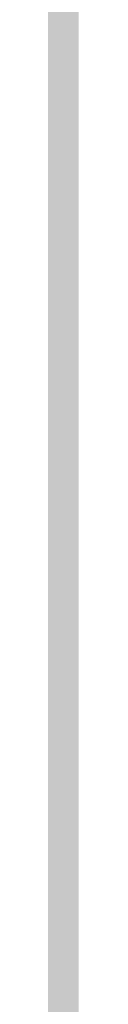
# Model space of a CAD drawing. Units: inches. Extents: x 2083 to 3317, y 1141 to 2115.
# Tile 174 of 256: x 3126.9594 to 3126.95969, y 1263.27402 to 1263.29018. Entities that reach past the tile are written whole.
import ezdxf

# ---------------------------------------------------------------- set-up
doc = ezdxf.new("R2010")
doc.units = ezdxf.units.IN
doc.layers.add('A-ANNO-DIMS', color=2, linetype='Continuous', lineweight=18)
doc.layers.add('A-WALL-PATT', color=251, linetype='Continuous', lineweight=13, true_color=0x636466)
doc.styles.get("Standard").update_dxf_attribs({"font": 'arial.ttf'})
doc.dimstyles.new('ISO-25', dxfattribs={"dimtxt": 12, "dimasz": 12, "dimexe": 1.25, "dimexo": 0.625, "dimtad": 1, "dimlunit": 3, "dimtxsty": 'Standard', "dimcen": 2.5, "dimadec": 0, "dimazin": 0, "dimtfac": 1, "dimtmove": 0, "dimatfit": 3, "dimfxl": 1, "dimarcsym": 0})

# ---------------------------------------------------------------- blocks, each defined once
blk = doc.blocks.new('*D26')
at = {"layer": 'A-ANNO-DIMS', "color": 0, "lineweight": -2, "transparency": 16777216}
for p, q in [((3088.985844, 1274.915092), (3088.985844, 1270.951963)), ((3111.240037, 1274.915092), (3111.240037, 1270.951963)), ((3076.985844, 1272.201963), (2840.262447, 1272.201963)), ((3111.240037, 1272.201963), (3088.985844, 1272.201963)), ((3123.240037, 1272.201963), (3135.240037, 1272.201963))]:
    blk.add_line(p, q, dxfattribs=at)
at = {"layer": 'A-ANNO-DIMS', "color": 0, "transparency": 16777216}
for points in [[(3076.985844, 1274.201963), (3076.985844, 1270.201963), (3088.985844, 1272.201963)], [(3123.240037, 1274.201963), (3123.240037, 1270.201963), (3111.240037, 1272.201963)]]:
    blk.add_solid(points, dxfattribs=at)
at = {"layer": 'Defpoints', "color": 0, "transparency": 16777216}
for p in [(3088.985844, 1275.540092), (3111.240037, 1275.540092), (3088.985844, 1272.201963)]:
    blk.add_point(p, dxfattribs=at)
at = {"layer": 'A-ANNO-DIMS', "color": 0, "transparency": 16777216, "insert": (2952.624146, 1279.031602), "char_height": 12, "attachment_point": 5}
blk.add_mtext('NIGHTSTAND 1\'-10 1/2" TYP.', dxfattribs=at)
blk = doc.blocks.new('*D27')
at = {"layer": 'A-ANNO-DIMS', "color": 0, "lineweight": -2, "transparency": 16777216}
for p, q in [((3114.578165, 1309.794285), (3114.578165, 1321.794285)), ((3111.865037, 1297.794285), (3115.828165, 1297.794285)), ((3114.578165, 1297.794285), (3114.578165, 1275.540092)), ((3111.865037, 1275.540092), (3115.828165, 1275.540092)), ((3114.578165, 1263.540092), (3114.578165, 1140.988591))]:
    blk.add_line(p, q, dxfattribs=at)
at = {"layer": 'A-ANNO-DIMS', "color": 0, "transparency": 16777216}
for points in [[(3112.578165, 1309.794285), (3116.578165, 1309.794285), (3114.578165, 1297.794285)], [(3112.578165, 1263.540092), (3116.578165, 1263.540092), (3114.578165, 1275.540092)]]:
    blk.add_solid(points, dxfattribs=at)
at = {"layer": 'Defpoints', "color": 0, "transparency": 16777216}
for p in [(3111.240037, 1297.794285), (3111.240037, 1275.540092), (3114.578165, 1275.540092)]:
    blk.add_point(p, dxfattribs=at)
at = {"layer": 'A-ANNO-DIMS', "color": 0, "transparency": 16777216, "insert": (3107.748527, 1196.264342), "char_height": 12, "attachment_point": 5, "rotation": 90}
blk.add_mtext('1\'-10 1/2" TYP.', dxfattribs=at)

msp = doc.modelspace()

# ---------------------------------------------------------------- hatches: boundary and pattern name
at = {"layer": 'A-WALL-PATT'}
h = msp.add_hatch(color=256, dxfattribs=at)
h.dxf.hatch_style = 1
h.paths.add_polyline_path([(3126.959783, 2020.76136), (2748.959783, 2020.76136), (2604.959783, 2020.76136), (2226.959783, 2020.76136), (2226.959783, 1702.76136), (2466.959783, 1702.76136), (2466.959783, 1582.76136), (2418.959783, 1582.76136), (2418.959783, 1477.76136), (2226.959783, 1477.76136), (2226.959783, 1263.26136), (2544.959783, 1263.26136), (2544.959783, 1411.76136), (2604.959783, 1411.76136), (2685.959783, 1411.76136), (2685.959783, 1420.76136), (2604.959783, 1420.76136), (2604.959783, 1573.76136), (2604.959783, 1702.76136), (2604.959783, 2011.76136), (2748.959783, 2011.76136), (2748.959783, 1702.76136), (2862.959783, 1702.76136), (2862.959783, 1621.76136), (2871.959783, 1621.76136), (2871.959783, 1702.76136), (2883.959783, 1702.76136), (2883.959783, 1706.939459, -0.026459), (2883.959783, 1711.76136), (2757.959783, 1711.76136), (2757.959783, 1807.76136), (2787.959783, 1807.76136), (2787.959783, 1812.26136), (2757.959783, 1812.26136), (2757.959783, 2011.76136), (2877.959783, 2011.76136), (2877.959783, 1812.26136), (2847.959783, 1812.26136), (2847.959783, 1807.76136), (2889.835742, 1807.76136), (2889.835742, 1812.26136), (2882.459783, 1812.26136), (2882.459783, 2011.76136), (3117.959783, 2011.76136), (3117.959783, 1812.26136), (2937.835742, 1812.26136), (2937.835742, 1807.76136), (2995.709783, 1807.76136), (2995.709783, 1796.117666), (3000.209783, 1796.117666), (3000.209783, 1807.76136), (3117.959783, 1807.76136), (3117.959783, 1711.76136), (3000.209783, 1711.76136), (3000.209783, 1760.117666), (2998.572705, 1760.117666, -0.020711), (2995.709783, 1760.117666), (2995.709783, 1711.76136), (2931.959783, 1711.76136), (2931.959783, 1702.76136), (3126.959783, 1702.76136)])
h.paths.add_polyline_path([(2471.459783, 2011.76136), (2471.459783, 1810.01136), (2462.716936, 1810.01136), (2462.716936, 1805.51136), (2505.959783, 1805.51136), (2505.959783, 1810.01136), (2475.959783, 1810.01136), (2475.959783, 2011.76136), (2595.959783, 2011.76136), (2595.959783, 1810.01136), (2565.959783, 1810.01136), (2565.959783, 1805.51136), (2595.959783, 1805.51136), (2595.959783, 1711.76136), (2235.959783, 1711.76136), (2235.959783, 1805.51136), (2353.709783, 1805.51136), (2353.709783, 1796.054162), (2358.209783, 1796.054162), (2358.209783, 1805.51136), (2414.716936, 1805.51136), (2414.716936, 1810.01136), (2235.959783, 1810.01136), (2235.959783, 2011.76136)], flags=16)
h.paths.add_polyline_path([(2270.204734, 1994.610008), (2270.204734, 1970.610008), (2246.204734, 1970.610008), (2246.204734, 1994.610008)], flags=0)
edge = h.paths.add_edge_path(flags=0)
edge.add_ellipse((2332.027391, 1899.798176), major_axis=(-3.042994, 3.042994), ratio=0.16825245, start_angle=-161.332166, end_angle=-156.307114, ccw=False)
edge.add_ellipse((2333.082037, 1898.74353), major_axis=(-1.054646, 1.054646), ratio=0.4535321, start_angle=-123.371019, end_angle=-94.159107)
edge = h.paths.add_edge_path(flags=0)
edge.add_ellipse((2332.027391, 1968.87629), major_axis=(3.042994, 3.042994), ratio=0.16825245, start_angle=18.667834, end_angle=23.692886)
edge.add_spline(control_points=[(2332.925596, 1970.691105), (2332.226768, 1970.3361), (2330.893709, 1969.658905), (2328.41308, 1970.932138), (2327.203934, 1967.748712), (2324.709596, 1969.955589), (2322.532822, 1967.012354), (2320.012846, 1971.295812), (2317.680308, 1968.157845), (2316.040526, 1967.102047), (2315.426904, 1966.809602)], knot_values=[0, 0, 0, 0, 2.267059, 4.324559, 6.685584, 8.878641, 11.121502, 14.300359, 17.755284, 19.732645, 19.732645, 19.732645, 19.732645], degree=3, periodic=0)
edge.add_ellipse((2332.027391, 1968.87629), major_axis=(3.042994, 3.042994), ratio=0.16825245, start_angle=18.667834, end_angle=23.692886, ccw=False)
edge.add_ellipse((2333.082037, 1969.930936), major_axis=(1.054646, 1.054646), ratio=0.4535321, start_angle=56.628981, end_angle=85.840893, ccw=False)
edge = h.paths.add_edge_path(flags=0)
edge.add_spline(control_points=[(2296.428287, 1967.987908), (2293.627804, 1965.336314), (2287.703624, 1959.727094), (2299.74386, 1949.995699), (2294.532591, 1935.668528), (2290.573228, 1920.603512), (2293.394124, 1909.973691), (2296.185407, 1904.966543)], knot_values=[0.099185, 0.099185, 0.099185, 0.099185, 0.345301, 0.619822, 0.982653, 1.386093, 1.810555, 1.810555, 1.810555, 1.810555], degree=3, periodic=0)
edge.add_spline(control_points=[(2296.185407, 1904.966543), (2297.383582, 1902.6193), (2298.000969, 1901.949312), (2298.55297, 1901.468155)], knot_values=[0.006246, 0.006246, 0.006246, 0.006246, 0.055476, 0.055476, 0.055476, 0.055476], degree=3, periodic=0)
edge.add_spline(control_points=[(2298.55297, 1901.468155), (2297.258612, 1900.923224), (2295.225294, 1900.232126), (2293.060229, 1900.614205), (2292.101423, 1900.788415), (2292.089578, 1900.790568)], knot_values=[0.312835, 0.312835, 0.312835, 0.312835, 0.40178, 0.474987, 0.475903, 0.475903, 0.475903, 0.475903], degree=3, periodic=0)
edge.add_arc((2292.793646, 1904.664109), 3.937008, 215.420897, 259.698179, ccw=False)
edge.add_spline(control_points=[(2289.585314, 1902.382304), (2289.476652, 1902.535087), (2289.36848, 1902.688035), (2289.260865, 1902.84117)], knot_values=[0.102872, 0.102872, 0.102872, 0.102872, 0.116896, 0.116896, 0.116896, 0.116896], degree=3, periodic=0)
edge.add_spline(control_points=[(2289.260865, 1902.84117), (2288.686604, 1902.550192), (2287.640048, 1902.019902), (2285.881337, 1901.873954), (2283.852972, 1901.504352), (2281.719987, 1899.710538), (2278.466991, 1899.492942), (2276.157136, 1901.883202), (2272.258953, 1899.804071), (2267.777605, 1901.843183), (2262.243882, 1900.184033), (2257.414927, 1901.782061), (2254.318374, 1900.72612), (2253.178285, 1900.337343)], knot_values=[0, 0, 0, 0, 1.907977, 3.477176, 5.261074, 7.972851, 11.680248, 13.717921, 16.939592, 22.789562, 27.502503, 33.595215, 37.145618, 37.145618, 37.145618, 37.145618], degree=3, periodic=0)
edge.add_line((2253.178285, 1900.337343), (2250.24424, 1902.84117))
edge.add_line((2250.24424, 1902.84117), (2250.24424, 1965.833296))
edge.add_line((2250.24424, 1965.833296), (2253.178285, 1968.337123))
edge.add_spline(control_points=[(2253.178285, 1968.337123), (2254.318374, 1967.948346), (2257.414927, 1966.892405), (2262.243882, 1968.490433), (2267.777605, 1966.831283), (2271.52673, 1968.537217), (2273.875914, 1967.828289), (2274.206701, 1967.727642)], knot_values=[0, 0, 0, 0, 0.09018, 0.244935, 0.364644, 0.513233, 0.537855, 0.537855, 0.537855, 0.537855], degree=3, periodic=0)
edge.add_arc((2274.352887, 1963.793349), 3.937008, 72.051134, 92.127949, ccw=False)
edge.add_arc((2281.296933, 1985.230003), 18.596298, 252.0511336, 288.5657217)
edge.add_arc((2292.316717, 1956.02888), 12.646081, 71.0267879, 113.7782184, ccw=False)
edge = h.paths.add_edge_path(flags=0)
edge.add_spline(control_points=[(2274.899415, 1951.856195), (2275.066156, 1951.616592), (2275.232687, 1951.376588), (2275.397987, 1951.135855)], knot_values=[1.409916, 1.409916, 1.409916, 1.409916, 1.43159, 1.43159, 1.43159, 1.43159], degree=3, periodic=0)
edge.add_spline(control_points=[(2275.397987, 1951.135855), (2275.792106, 1950.561885), (2276.179231, 1949.983774), (2276.545546, 1949.397103)], knot_values=[1.358238, 1.358238, 1.358238, 1.358238, 1.409916, 1.409916, 1.409916, 1.409916], degree=3, periodic=0)
edge.add_line((2276.545546, 1949.397103), (2277.437289, 1947.862185))
edge.add_spline(control_points=[(2277.437289, 1947.862185), (2276.303834, 1945.673115), (2274.639698, 1942.426882), (2274.631615, 1938.0939), (2272.799124, 1930.85155), (2274.356426, 1943.897046), (2275.947681, 1947.923356), (2276.545546, 1949.397103)], knot_values=[0.005632, 0.005632, 0.005632, 0.005632, 0.186014, 0.266002, 0.357087, 0.59639, 0.739732, 0.739732, 0.739732, 0.739732], degree=3, periodic=0)
edge.add_spline(control_points=[(2276.545546, 1949.397103), (2276.179231, 1949.983774), (2275.792106, 1950.561885), (2275.397987, 1951.135855)], knot_values=[1.358238, 1.358238, 1.358238, 1.358238, 1.409916, 1.409916, 1.409916, 1.409916], degree=3, periodic=0)
edge.add_spline(control_points=[(2275.397987, 1951.135855), (2274.9425, 1950.080452), (2274.20776, 1948.025272), (2273.934602, 1944.851477), (2272.468534, 1937.627489), (2273.466216, 1945.696466), (2274.700615, 1951.059472), (2274.899415, 1951.856195)], knot_values=[0.104364, 0.104364, 0.104364, 0.104364, 0.189636, 0.269624, 0.36071, 0.600013, 0.644622, 0.644622, 0.644622, 0.644622], degree=3, periodic=0)
h.paths.add_polyline_path([(2269.167514, 1963.127573, -0.357527), (2268.170633, 1960.97637, -0.092561), (2268.170633, 1939.436325, -0.357527), (2269.167514, 1937.285122, -0.357527), (2267.01631, 1938.282002, -0.164785), (2254.685581, 1938.282002, -0.357527), (2252.534378, 1937.285122, -0.357527), (2253.531259, 1939.436325, -0.092561), (2253.531259, 1960.97637, -0.357527), (2252.534378, 1963.127573, -0.357527), (2254.685581, 1962.130692, -0.164785), (2267.01631, 1962.130692, -0.357527)], flags=0)
h.paths.add_polyline_path([(2248.874068, 1967.8018), (2248.874068, 1957.02771), (2249.457783, 1957.02771), (2249.457783, 1911.646756), (2248.874068, 1911.646756), (2248.874068, 1900.872666), (2246.511863, 1900.872666, 0.197327), (2244.149658, 1902.456873), (2244.149658, 1966.217592, 0.197327), (2246.511863, 1967.8018)], flags=0)
h.paths.add_polyline_path([(2269.167514, 1931.389344, -0.357527), (2268.170633, 1929.238141, -0.092561), (2268.170633, 1907.698096, -0.357527), (2269.167514, 1905.546893, -0.357527), (2267.01631, 1906.543774, -0.164785), (2254.685581, 1906.543774, -0.357527), (2252.534378, 1905.546893, -0.357527), (2253.531259, 1907.698096, -0.092561), (2253.531259, 1929.238141, -0.357527), (2252.534378, 1931.389344, -0.357527), (2254.685581, 1930.392463, -0.164785), (2267.01631, 1930.392463, -0.357527)], flags=0)
edge = h.paths.add_edge_path(flags=0)
edge.add_spline(control_points=[(2276.196858, 1906.723702), (2276.168144, 1909.028928), (2276.114049, 1913.371852), (2270.598417, 1924.924978), (2273.905175, 1919.012779), (2275.921711, 1916.262063), (2275.47457, 1912.402149), (2277.257874, 1910.380621), (2276.696044, 1908.225036), (2276.646218, 1906.813023), (2276.617825, 1906.008407)], knot_values=[0, 0, 0, 0, 8.61026, 16.221274, 18.843057, 23.804898, 27.440828, 29.356102, 31.203478, 33.650687, 33.650687, 33.650687, 33.650687], degree=3, periodic=0)
edge.add_spline(control_points=[(2276.617825, 1906.008407), (2276.623313, 1905.624144), (2276.497738, 1904.628661), (2275.441779, 1903.854725), (2274.937314, 1903.08045), (2274.85908, 1902.84117)], knot_values=[0.156488, 0.156488, 0.156488, 0.156488, 0.184398, 0.231376, 0.250598, 0.250598, 0.250598, 0.250598], degree=3, periodic=0)
edge.add_line((2274.85908, 1902.84117), (2276.50598, 1902.84117))
edge.add_spline(control_points=[(2276.50598, 1902.84117), (2276.788308, 1903.08494), (2277.665071, 1904.125196), (2278.249538, 1904.340738), (2277.653872, 1908.527387), (2278.15567, 1906.227808), (2278.100464, 1905.285948), (2278.846675, 1904.069005), (2277.856785, 1903.414948), (2277.874191, 1902.99105), (2277.903562, 1902.84117)], knot_values=[0.059574, 0.059574, 0.059574, 0.059574, 0.080753, 0.103741, 0.16972, 0.176036, 0.207137, 0.240474, 0.262341, 0.27366, 0.27366, 0.27366, 0.27366], degree=3, periodic=0)
edge.add_line((2277.903562, 1902.84117), (2280.029825, 1902.84117))
edge.add_spline(control_points=[(2280.029825, 1902.84117), (2279.888221, 1903.088398), (2279.499257, 1903.981551), (2280.152284, 1905.939349), (2278.103615, 1909.657757), (2279.762395, 1907.185285), (2280.3279, 1904.874861), (2280.485109, 1903.48959), (2281.463269, 1903.249432), (2281.758343, 1902.936497), (2281.834036, 1902.84117)], knot_values=[0.013856, 0.013856, 0.013856, 0.013856, 0.034874, 0.088867, 0.107879, 0.126738, 0.158714, 0.193757, 0.217487, 0.226722, 0.226722, 0.226722, 0.226722], degree=3, periodic=0)
edge.add_spline(control_points=[(2281.834036, 1902.84117), (2281.787535, 1902.826703), (2281.647022, 1902.782988), (2281.395527, 1902.85949), (2281.088077, 1902.985242), (2280.720683, 1903.060902), (2280.333451, 1903.025726), (2280.124767, 1902.898879), (2280.029825, 1902.84117)], knot_values=[0, 0, 0, 0, 0.14413, 0.435517, 0.749276, 1.153046, 1.548371, 1.878348, 1.878348, 1.878348, 1.878348], degree=3, periodic=0)
edge.add_line((2280.029825, 1902.84117), (2277.903562, 1902.84117))
edge.add_spline(control_points=[(2277.903562, 1902.84117), (2277.892855, 1902.795855), (2277.865396, 1902.679637), (2277.607479, 1902.687483), (2277.27405, 1902.8007), (2276.837921, 1902.619775), (2276.583807, 1902.789261), (2276.50598, 1902.84117)], knot_values=[0, 0, 0, 0, 0.127189, 0.326199, 0.628009, 1.24357, 1.515331, 1.515331, 1.515331, 1.515331], degree=3, periodic=0)
edge.add_line((2276.50598, 1902.84117), (2274.85908, 1902.84117))
edge.add_spline(control_points=[(2274.85908, 1902.84117), (2274.814437, 1902.898587), (2274.72513, 1903.013446), (2274.493477, 1903.118968), (2274.244285, 1902.960539), (2273.937121, 1903.184942), (2273.614039, 1902.983143), (2273.408316, 1902.883045), (2273.322254, 1902.84117)], knot_values=[0, 0, 0, 0, 0.21843, 0.436957, 0.687977, 0.990379, 1.398396, 1.69185, 1.69185, 1.69185, 1.69185], degree=3, periodic=0)
edge.add_spline(control_points=[(2273.322254, 1902.84117), (2273.61674, 1903.445692), (2274.273998, 1904.538253), (2276.027239, 1904.573702), (2276.206963, 1906.583637), (2276.196858, 1906.723702)], knot_values=[0.012227, 0.012227, 0.012227, 0.012227, 0.059472, 0.106218, 0.134458, 0.134458, 0.134458, 0.134458], degree=3, periodic=0)
h.paths.add_polyline_path([(2270.776054, 1897.789828), (2270.776054, 1873.789828), (2246.776054, 1873.789828), (2246.776054, 1897.789828)], flags=0)
h.paths.add_polyline_path([(2353.709783, 1760.005059), (2353.709783, 1760.054162), (2358.209783, 1760.054162, -0.033729)], flags=0)
h.paths.add_polyline_path([(2321.819119, 1737.529186), (2341.995327, 1737.529186, -0.414214), (2343.203273, 1736.321241), (2343.203273, 1721.020596, -0.414214), (2341.995327, 1719.812651), (2321.819119, 1719.812651, -0.414214), (2320.611173, 1721.020596), (2320.611173, 1736.321241, -0.414214)], flags=0)
h.paths.add_polyline_path([(2324.23501, 1736.321241), (2339.579436, 1736.321241, -0.414214), (2341.995327, 1733.905349), (2341.995327, 1725.44973, -0.414214), (2339.579436, 1723.033839), (2333.680588, 1723.033839), (2333.845317, 1722.045467, -0.870646), (2335.425399, 1721.825893, -0.767327), (2333.922694, 1721.423245), (2331.291024, 1721.423245, -0.767327), (2329.788319, 1721.825893, -0.870646), (2331.368401, 1722.045467), (2331.53313, 1723.033839), (2324.23501, 1723.033839, -0.414214), (2321.819119, 1725.44973), (2321.819119, 1733.905349, -0.414214)], flags=0)
h.paths.add_polyline_path([(2570.483789, 1928.615444), (2589.683789, 1928.615444), (2590.168829, 1928.615444), (2590.168829, 1904.993397), (2570.483789, 1904.993397)], flags=0)
h.paths.add_polyline_path([(2574.447324, 1927.263822, -1), (2572.828836, 1927.263822, -1)], flags=0)
h.paths.add_polyline_path([(2573.089867, 1926.940877), (2573.925032, 1927.776042), (2574.147743, 1927.553332), (2573.312577, 1926.718166)], flags=0)
h.paths.add_polyline_path([(2578.779065, 1919.729618, -1), (2571.591663, 1919.729618, -1)], flags=0)
h.paths.add_polyline_path([(2578.385364, 1919.729618, -1), (2571.985364, 1919.729618, -1)], flags=0)
h.paths.add_polyline_path([(2331.595764, 1729.476216, -1), (2333.617954, 1729.476216, -1)], flags=0)
h.paths.add_polyline_path([(2578.034228, 1927.263822, -1), (2576.41574, 1927.263822, -1)], flags=0)
h.paths.add_polyline_path([(2576.688851, 1927.531089), (2576.911562, 1927.753799), (2577.746728, 1926.918634), (2577.524017, 1926.695923)], flags=0)
h.paths.add_polyline_path([(2578.139065, 1909.859539, -1), (2572.231663, 1909.859539, -1)], flags=0)
h.paths.add_polyline_path([(2577.745364, 1909.859539, -1), (2572.625364, 1909.859539, -1)], flags=0)
h.paths.add_polyline_path([(2583.797718, 1927.263822, -1), (2582.179229, 1927.263822, -1)], flags=0)
h.paths.add_polyline_path([(2582.718649, 1927.753799), (2583.553814, 1926.918634), (2583.331103, 1926.695923), (2582.495938, 1927.531089)], flags=0)
h.paths.add_polyline_path([(2582.495938, 1927.531089), (2582.718649, 1927.753799), (2583.553814, 1926.918634), (2583.331103, 1926.695923)], flags=0)
h.paths.add_polyline_path([(2587.739065, 1920.529618, -1), (2581.831663, 1920.529618, -1)], flags=0)
h.paths.add_polyline_path([(2587.345364, 1920.529618, -1), (2582.225364, 1920.529618, -1)], flags=0)
h.paths.add_polyline_path([(2587.384622, 1927.263822, -1), (2585.766133, 1927.263822, -1)], flags=0)
h.paths.add_polyline_path([(2586.081993, 1926.980247), (2586.917158, 1927.815412), (2587.139869, 1927.592702), (2586.304703, 1926.757536)], flags=0)
h.paths.add_polyline_path([(2588.379065, 1910.659539, -1), (2581.191663, 1910.659539, -1)], flags=0)
h.paths.add_polyline_path([(2587.985364, 1910.659539, -1), (2581.585364, 1910.659539, -1)], flags=0)
h.paths.add_polyline_path([(2417.167729, 1729.477895), (2437.343937, 1729.477895, -0.414214), (2438.551883, 1728.26995), (2438.551883, 1712.969306, -0.414214), (2437.343937, 1711.76136), (2417.167729, 1711.76136, -0.414214), (2415.959783, 1712.969306), (2415.959783, 1728.26995, -0.414214)], flags=0)
h.paths.add_polyline_path([(2419.58362, 1728.26995), (2434.928046, 1728.26995, -0.414214), (2437.343937, 1725.854059), (2437.343937, 1717.39844, -0.414214), (2434.928046, 1714.982548), (2429.029199, 1714.982548), (2429.193927, 1713.994176, -0.870646), (2430.774009, 1713.774603, -0.767327), (2429.271304, 1713.371954), (2426.639634, 1713.371954, -0.767327), (2425.136929, 1713.774603, -0.870646), (2426.717011, 1713.994176), (2426.88174, 1714.982548), (2419.58362, 1714.982548, -0.414214), (2417.167729, 1717.39844), (2417.167729, 1725.854059, -0.414214)], flags=0)
h.paths.add_polyline_path([(2419.58362, 1728.26995), (2434.928046, 1728.26995, -0.414214), (2437.343937, 1725.854059), (2437.343937, 1717.39844, -0.414214), (2434.928046, 1714.982548), (2429.029199, 1714.982548), (2428.358118, 1719.009034), (2427.552821, 1719.009034), (2426.88174, 1714.982548), (2419.58362, 1714.982548, -0.414214), (2417.167729, 1717.39844), (2417.167729, 1725.854059, -0.414214)], flags=0)
h.paths.add_polyline_path([(2426.944374, 1721.424925, -1), (2428.966564, 1721.424925, -1)], flags=0)
h.paths.add_polyline_path([(2475.959783, 1702.76136), (2595.959783, 1702.76136), (2595.959783, 1582.76136), (2475.959783, 1582.76136)], flags=16)
h.paths.add_polyline_path([(2427.959783, 1573.76136), (2595.959783, 1573.76136), (2595.959783, 1468.76136), (2595.959783, 1420.76136), (2384.459783, 1420.76136), (2384.459783, 1468.76136), (2427.959783, 1468.76136)], flags=16)
h.paths.add_polyline_path([(2379.959783, 1468.76136), (2379.959783, 1420.76136), (2235.959783, 1420.76136), (2235.959783, 1468.76136)], flags=16)
h.paths.add_polyline_path([(2317.815996, 1466.695767), (2337.992205, 1466.695767, -0.414214), (2339.20015, 1465.487821), (2339.20015, 1450.187177, -0.414214), (2337.992205, 1448.979232), (2317.815996, 1448.979232, -0.414214), (2316.608051, 1450.187177), (2316.608051, 1465.487821, -0.414214)], flags=0)
h.paths.add_polyline_path([(2320.231887, 1465.487821), (2335.576313, 1465.487821, -0.414214), (2337.992205, 1463.07193), (2337.992205, 1454.616311, -0.414214), (2335.576313, 1452.20042), (2329.677466, 1452.20042), (2329.842195, 1451.212047, -0.870646), (2331.422276, 1450.992474, -0.767327), (2329.919571, 1450.589826), (2327.287902, 1450.589826, -0.767327), (2325.785197, 1450.992474, -0.870646), (2327.365278, 1451.212047), (2327.530007, 1452.20042), (2320.231887, 1452.20042, -0.414214), (2317.815996, 1454.616311), (2317.815996, 1463.07193, -0.414214)], flags=0)
h.paths.add_polyline_path([(2320.231887, 1465.487821), (2335.576313, 1465.487821, -0.414214), (2337.992205, 1463.07193), (2337.992205, 1454.616311, -0.414214), (2335.576313, 1452.20042), (2329.677466, 1452.20042), (2329.006385, 1456.226905), (2328.201088, 1456.226905), (2327.530007, 1452.20042), (2320.231887, 1452.20042, -0.414214), (2317.815996, 1454.616311), (2317.815996, 1463.07193, -0.414214)], flags=0)
h.paths.add_polyline_path([(2327.592641, 1458.642796, -1), (2329.614832, 1458.642796, -1)], flags=0)
h.paths.add_polyline_path([(2244.411744, 1433.340453), (2241.920945, 1433.340453, -0.414214), (2240.017856, 1435.243542), (2240.017856, 1440.952808, -0.414211), (2241.920925, 1442.855897), (2244.411744, 1442.855897, -1.976472)], flags=0)
h.paths.add_polyline_path([(2245.356888, 1434.397536, -0.414214), (2245.356888, 1441.798814, -2.144098)], flags=0)
h.paths.add_polyline_path([(2535.959783, 1416.26136), (2535.959783, 1272.26136), (2235.959783, 1272.26136), (2235.959783, 1416.26136)], flags=16)
h.paths.add_polyline_path([(2260.119561, 1384.292841), (2260.119561, 1362.038649), (2237.865369, 1362.038649), (2237.865369, 1384.292841)], flags=0)
edge = h.paths.add_edge_path(flags=0)
edge.add_line((2318.251847, 1362.093298), (2318.145797, 1362.000973))
edge.add_ellipse((2317.445116, 1360.431044), major_axis=(2.82164, 2.82164), ratio=0.16825245, start_angle=18.667834, end_angle=20.948127, ccw=False)
edge.add_ellipse((2318.423045, 1361.408974), major_axis=(0.977929, 0.977929), ratio=0.4535321, start_angle=56.628981, end_angle=70.226201, ccw=False)
edge = h.paths.add_edge_path(flags=0)
edge.add_line((2319.10737, 1295.571078), (2319.015044, 1295.677128))
edge.add_ellipse((2317.445116, 1296.377809), major_axis=(-2.82164, 2.82164), ratio=0.16825245, start_angle=-161.332166, end_angle=-159.051873, ccw=False)
edge.add_ellipse((2318.423045, 1295.39988), major_axis=(-0.977929, 0.977929), ratio=0.4535321, start_angle=-123.371019, end_angle=-109.773799)
edge = h.paths.add_edge_path(flags=0)
edge.add_spline(control_points=[(2284.210349, 1301.170219), (2284.580688, 1300.444719), (2284.891189, 1299.892024), (2285.159553, 1299.461018)], knot_values=[0.039066, 0.039066, 0.039066, 0.039066, 0.055476, 0.055476, 0.055476, 0.055476], degree=3, periodic=0)
edge.add_line((2285.159553, 1299.461018), (2284.210349, 1301.170219))
edge = h.paths.add_edge_path(flags=0)
edge.add_line((2280.412458, 1297.298013), (2283.369991, 1297.036122))
edge.add_line((2283.369991, 1297.036122), (2286.40569, 1297.92631))
edge.add_spline(control_points=[(2286.40569, 1297.92631), (2285.305487, 1297.463119), (2284.344777, 1297.129151), (2283.369991, 1297.036122)], knot_values=[0.394369, 0.394369, 0.394369, 0.394369, 0.475903, 0.475903, 0.475903, 0.475903], degree=3, periodic=0)
edge.add_spline(control_points=[(2283.369991, 1297.036122), (2283.28139, 1297.027666), (2282.316289, 1296.957336), (2281.312502, 1297.134479), (2280.423441, 1297.296016), (2280.412458, 1297.298013)], knot_values=[0.312835, 0.312835, 0.312835, 0.312835, 0.320246, 0.393453, 0.394369, 0.394369, 0.394369, 0.394369], degree=3, periodic=0)
edge = h.paths.add_edge_path(flags=0)
edge.add_line((2284.435561, 1359.607285), (2280.446291, 1355.328047))
edge.add_line((2280.446291, 1355.328047), (2279.579987, 1351.017754))
edge.add_line((2279.579987, 1351.017754), (2282.412974, 1346.580433))
edge.add_spline(control_points=[(2282.412974, 1346.580433), (2283.153331, 1345.589236), (2284.252896, 1344.028897), (2284.801037, 1342.387167), (2284.935162, 1341.805544)], knot_values=[1.240098, 1.240098, 1.240098, 1.240098, 1.332892, 1.382712, 1.382712, 1.382712, 1.382712], degree=3, periodic=0)
edge.add_spline(control_points=[(2284.935162, 1341.805544), (2285.319108, 1340.1406), (2285.233029, 1338.409204), (2284.909938, 1336.654122)], knot_values=[1.097484, 1.097484, 1.097484, 1.097484, 1.240098, 1.240098, 1.240098, 1.240098], degree=3, periodic=0)
edge.add_spline(control_points=[(2284.909938, 1336.654122), (2284.586848, 1334.89904), (2284.026745, 1333.120272), (2283.462644, 1331.360585)], knot_values=[0.95487, 0.95487, 0.95487, 0.95487, 1.097484, 1.097484, 1.097484, 1.097484], degree=3, periodic=0)
edge.add_line((2283.462644, 1331.360585), (2281.890376, 1326.153357))
edge.add_line((2281.890376, 1326.153357), (2280.756259, 1321.056089))
edge.add_line((2280.756259, 1321.056089), (2280.299205, 1316.001977))
edge.add_line((2280.299205, 1316.001977), (2280.715933, 1310.950068))
edge.add_line((2280.715933, 1310.950068), (2282.028094, 1305.972137))
edge.add_line((2282.028094, 1305.972137), (2284.210349, 1301.170219))
edge.add_spline(control_points=[(2284.210349, 1301.170219), (2283.340731, 1302.730185), (2282.611904, 1304.336493), (2282.028094, 1305.972137)], knot_values=[0.099185, 0.099185, 0.099185, 0.099185, 0.241799, 0.241799, 0.241799, 0.241799], degree=3, periodic=0)
edge.add_spline(control_points=[(2282.028094, 1305.972137), (2281.444283, 1307.60778), (2281.005489, 1309.272759), (2280.715933, 1310.950068)], knot_values=[0.241799, 0.241799, 0.241799, 0.241799, 0.384413, 0.384413, 0.384413, 0.384413], degree=3, periodic=0)
edge.add_spline(control_points=[(2280.715933, 1310.950068), (2280.433241, 1312.587613), (2280.289386, 1314.276959), (2280.298894, 1315.962032), (2280.299205, 1316.001977)], knot_values=[0.384413, 0.384413, 0.384413, 0.384413, 0.523647, 0.527028, 0.527028, 0.527028, 0.527028], degree=3, periodic=0)
edge.add_spline(control_points=[(2280.299205, 1316.001977), (2280.312326, 1317.686955), (2280.477871, 1319.367926), (2280.756259, 1321.056089)], knot_values=[0.527028, 0.527028, 0.527028, 0.527028, 0.669642, 0.669642, 0.669642, 0.669642], degree=3, periodic=0)
edge.add_spline(control_points=[(2280.756259, 1321.056089), (2281.034648, 1322.744252), (2281.42588, 1324.439608), (2281.890376, 1326.153357)], knot_values=[0.669642, 0.669642, 0.669642, 0.669642, 0.812256, 0.812256, 0.812256, 0.812256], degree=3, periodic=0)
edge.add_spline(control_points=[(2281.890376, 1326.153357), (2282.264383, 1327.533251), (2282.78787, 1329.26181), (2283.352751, 1331.01778), (2283.462644, 1331.360585)], knot_values=[0.812256, 0.812256, 0.812256, 0.812256, 0.927087, 0.95487, 0.95487, 0.95487, 0.95487], degree=3, periodic=0)
edge.add_line((2283.462644, 1331.360585), (2284.909938, 1336.654122))
edge.add_line((2284.909938, 1336.654122), (2284.935162, 1341.805544))
edge.add_line((2284.935162, 1341.805544), (2282.412974, 1346.580433))
edge.add_spline(control_points=[(2282.412974, 1346.580433), (2281.275127, 1348.103792), (2280.078447, 1349.570318), (2279.579987, 1351.017754)], knot_values=[1.382712, 1.382712, 1.382712, 1.382712, 1.525326, 1.525326, 1.525326, 1.525326], degree=3, periodic=0)
edge.add_spline(control_points=[(2279.579987, 1351.017754), (2279.443282, 1351.414721), (2279.136312, 1352.856922), (2279.73519, 1354.290385), (2280.446291, 1355.328047)], knot_values=[1.525326, 1.525326, 1.525326, 1.525326, 1.564439, 1.667941, 1.667941, 1.667941, 1.667941], degree=3, periodic=0)
edge.add_spline(control_points=[(2280.446291, 1355.328047), (2281.426113, 1356.757835), (2282.930837, 1358.18256), (2284.435561, 1359.607285)], knot_values=[1.667941, 1.667941, 1.667941, 1.667941, 1.810555, 1.810555, 1.810555, 1.810555], degree=3, periodic=0)
edge.add_arc((2280.623075, 1348.518181), 11.72618, 71.0267879, 113.7782184)
edge.add_arc((2270.404892, 1375.595156), 17.243567, 252.0511336, 288.5657217, ccw=False)
edge.add_arc((2263.965969, 1355.717847), 3.650622, 72.051134, 92.127949)
edge.add_arc((2263.965969, 1355.717847), 3.650622, 92.127949, 177.98513)
edge.add_spline(control_points=[(2260.317604, 1355.846199), (2260.260417, 1354.220668), (2260.551278, 1350.186547), (2262.999344, 1346.766251), (2264.472741, 1344.649024)], knot_values=[1.43159, 1.43159, 1.43159, 1.43159, 1.564144, 1.770695, 1.770695, 1.770695, 1.770695], degree=3, periodic=0)
edge.add_line((2264.472741, 1344.649024), (2264.93559, 1343.98253))
edge.add_spline(control_points=[(2263.801044, 1340.248105), (2263.843238, 1340.514088), (2264.067244, 1341.756465), (2264.512693, 1343.002453), (2264.935047, 1343.981083)], knot_values=[0.53657, 0.53657, 0.53657, 0.53657, 0.559349, 0.644622, 0.644622, 0.644622, 0.644622], degree=3, periodic=0)
edge.add_spline(control_points=[(2264.935047, 1343.981083), (2265.117771, 1343.714975), (2265.298875, 1343.447906), (2265.476756, 1343.179365)], knot_values=[1.384077, 1.384077, 1.384077, 1.384077, 1.409916, 1.409916, 1.409916, 1.409916], degree=3, periodic=0)
edge.add_spline(control_points=[(2265.476756, 1343.179365), (2265.654637, 1342.910823), (2265.829296, 1342.64081), (2265.99913, 1342.368812)], knot_values=[1.358238, 1.358238, 1.358238, 1.358238, 1.384077, 1.384077, 1.384077, 1.384077], degree=3, periodic=0)
edge.add_line((2265.99913, 1342.368812), (2266.826006, 1340.945547))
edge.add_spline(control_points=[(2266.826006, 1340.945547), (2268.894401, 1337.089691), (2271.398173, 1325.843001), (2270.516164, 1310.568557), (2275.919376, 1301.860609), (2277.789511, 1299.19945)], knot_values=[0.116896, 0.116896, 0.116896, 0.116896, 0.472987, 1.050969, 1.313793, 1.313793, 1.313793, 1.313793], degree=3, periodic=0)
edge.add_spline(control_points=[(2277.789511, 1299.19945), (2277.839405, 1299.128452), (2277.889428, 1299.057498), (2277.939572, 1298.986584)], knot_values=[0.109884, 0.109884, 0.109884, 0.109884, 0.116896, 0.116896, 0.116896, 0.116896], degree=3, periodic=0)
edge.add_line((2277.939572, 1298.986584), (2277.788849, 1299.199114))
edge.add_spline(control_points=[(2277.788849, 1299.199114), (2277.256582, 1298.929414), (2276.28635, 1298.437902), (2275.039352, 1298.334419), (2274.38333, 1298.238895), (2274.215254, 1298.209338)], knot_values=[33.12187, 33.12187, 33.12187, 33.12187, 35.029056, 36.598255, 37.144827, 37.144827, 37.144827, 37.144827], degree=3, periodic=0)
edge.add_line((2274.215254, 1298.209338), (2273.073147, 1297.892961))
edge.add_spline(control_points=[(2273.073147, 1297.892961), (2272.322936, 1297.579784), (2271.039151, 1296.510508), (2269.248395, 1296.226062), (2268.4231, 1296.374654)], knot_values=[26.532584, 26.532584, 26.532584, 26.532584, 29.198919, 31.839101, 31.839101, 31.839101, 31.839101], degree=3, periodic=0)
edge.add_line((2268.4231, 1296.374654), (2263.878501, 1297.457534))
edge.add_spline(control_points=[(2263.878501, 1297.457534), (2263.556077, 1297.359435), (2261.860306, 1296.838694), (2260.23878, 1297.282407), (2258.933454, 1297.516461)], knot_values=[15.919551, 15.919551, 15.919551, 15.919551, 16.939592, 21.226067, 21.226067, 21.226067, 21.226067], degree=3, periodic=0)
edge.add_line((2258.933454, 1297.516461), (2254.055233, 1297.32901))
edge.add_spline(control_points=[(2254.055233, 1297.32901), (2253.755525, 1297.295815), (2252.113683, 1297.165174), (2250.461869, 1297.544221), (2249.129686, 1297.667882)], knot_values=[5.306517, 5.306517, 5.306517, 5.306517, 6.276435, 10.613034, 10.613034, 10.613034, 10.613034], degree=3, periodic=0)
edge.add_line((2249.129686, 1297.667882), (2244.33165, 1296.877756))
edge.add_line((2244.33165, 1296.877756), (2241.611033, 1299.19945))
edge.add_line((2241.611033, 1299.19945), (2241.611033, 1357.609404))
edge.add_line((2241.611033, 1357.609404), (2244.33165, 1359.931097))
edge.add_line((2244.33165, 1359.931097), (2252.728823, 1359.542692))
edge.add_spline(control_points=[(2252.728823, 1359.542692), (2252.870939, 1359.54644), (2253.30574, 1359.548172), (2253.739845, 1359.514274), (2254.031742, 1359.482426)], knot_values=[0.233291, 0.233291, 0.233291, 0.233291, 0.244935, 0.268927, 0.268927, 0.268927, 0.268927], degree=3, periodic=0)
edge.add_line((2254.031742, 1359.482426), (2259.58719, 1359.41639))
edge.add_spline(control_points=[(2259.58719, 1359.41639), (2260.677068, 1359.628503), (2262.073197, 1359.897003), (2263.523692, 1359.459278), (2263.830417, 1359.365952)], knot_values=[0.422516, 0.422516, 0.422516, 0.422516, 0.513233, 0.537855, 0.537855, 0.537855, 0.537855], degree=3, periodic=0)
edge.add_arc((2263.965969, 1355.717847), 3.650622, 72.051134, 92.127949, ccw=False)
edge.add_arc((2270.404892, 1375.595156), 17.243567, 252.0511336, 288.5657217)
edge.add_arc((2280.623075, 1348.518181), 11.72618, 71.0267879, 113.7782184, ccw=False)
h.paths.add_polyline_path([(2240.34053, 1359.434715), (2240.34053, 1349.444353), (2240.881785, 1349.444353), (2240.881785, 1307.3645), (2240.34053, 1307.3645), (2240.34053, 1297.374138), (2238.150157, 1297.374138, 0.197327), (2235.959783, 1298.843108), (2235.959783, 1357.965746, 0.197327), (2238.150157, 1359.434715)], flags=0)
h.paths.add_polyline_path([(2259.15779, 1355.1005, -0.357527), (2258.233425, 1353.10578, -0.092561), (2258.233425, 1333.132601, -0.357527), (2259.15779, 1331.13788, -0.357527), (2257.16307, 1332.062246, -0.164785), (2245.729302, 1332.062246, -0.357527), (2243.734582, 1331.13788, -0.357527), (2244.658947, 1333.132601, -0.092561), (2244.658947, 1353.10578, -0.357527), (2243.734582, 1355.1005, -0.357527), (2245.729302, 1354.176135, -0.164785), (2257.16307, 1354.176135, -0.357527)], flags=0)
edge = h.paths.add_edge_path(flags=0)
edge.add_line((2265.99913, 1342.368812), (2266.826006, 1340.945547))
edge.add_line((2266.826006, 1340.945547), (2265.307557, 1337.814066))
edge.add_line((2265.307557, 1337.814066), (2264.358232, 1334.652939))
edge.add_line((2264.358232, 1334.652939), (2264.262012, 1333.799705))
edge.add_spline(control_points=[(2264.262012, 1333.799705), (2264.208357, 1333.187055), (2264.16206, 1332.365525), (2264.007144, 1331.413933), (2263.969049, 1331.201834)], knot_values=[0.464444, 0.464444, 0.464444, 0.464444, 0.516691, 0.531608, 0.531608, 0.531608, 0.531608], degree=3, periodic=0)
edge.add_spline(control_points=[(2263.969049, 1331.201834), (2263.774535, 1330.118873), (2263.42437, 1328.790839), (2263.25742, 1328.530652), (2263.234028, 1328.514612)], knot_values=[0.372682, 0.372682, 0.372682, 0.372682, 0.44885, 0.464444, 0.464444, 0.464444, 0.464444], degree=3, periodic=0)
edge.add_spline(control_points=[(2263.234028, 1328.514612), (2263.096382, 1328.420227), (2263.13117, 1329.301477), (2263.274953, 1330.615749)], knot_values=[0.280919, 0.280919, 0.280919, 0.280919, 0.372682, 0.372682, 0.372682, 0.372682], degree=3, periodic=0)
edge.add_spline(control_points=[(2263.274953, 1330.615749), (2263.418736, 1331.930022), (2263.671515, 1333.677318), (2263.969852, 1335.315027)], knot_values=[0.189157, 0.189157, 0.189157, 0.189157, 0.280919, 0.280919, 0.280919, 0.280919], degree=3, periodic=0)
edge.add_spline(control_points=[(2263.969852, 1335.315027), (2264.100496, 1336.032192), (2264.418783, 1337.621911), (2264.754848, 1338.86443), (2264.947419, 1339.491124)], knot_values=[0.097394, 0.097394, 0.097394, 0.097394, 0.137578, 0.189157, 0.189157, 0.189157, 0.189157], degree=3, periodic=0)
edge.add_spline(control_points=[(2264.947419, 1339.491124), (2265.290017, 1340.606055), (2265.644238, 1341.493996), (2265.99913, 1342.368812)], knot_values=[0.005632, 0.005632, 0.005632, 0.005632, 0.097394, 0.097394, 0.097394, 0.097394], degree=3, periodic=0)
h.paths.add_polyline_path([(2259.15779, 1325.670973, -0.357527), (2258.233425, 1323.676253, -0.092561), (2258.233425, 1303.703073, -0.357527), (2259.15779, 1301.708353, -0.357527), (2257.16307, 1302.632719, -0.164785), (2245.729302, 1302.632719, -0.357527), (2243.734582, 1301.708353, -0.357527), (2244.658947, 1303.703073, -0.092561), (2244.658947, 1323.676253, -0.357527), (2243.734582, 1325.670973, -0.357527), (2245.729302, 1324.746608, -0.164785), (2257.16307, 1324.746608, -0.357527)], flags=0)
edge = h.paths.add_edge_path(flags=0)
edge.add_spline(control_points=[(2261.708938, 1317.311421), (2261.679482, 1317.41758), (2261.761858, 1317.388535), (2262.490736, 1316.089873), (2262.962185, 1315.300897)], knot_values=[14.955861, 14.955861, 14.955861, 14.955861, 16.221274, 18.694826, 18.694826, 18.694826, 18.694826], degree=3, periodic=0)
edge.add_spline(control_points=[(2262.962185, 1315.300897), (2262.990437, 1315.253617), (2263.702096, 1314.067376), (2264.348983, 1313.127153), (2264.730054, 1312.164154)], knot_values=[18.694826, 18.694826, 18.694826, 18.694826, 18.843057, 22.433791, 22.433791, 22.433791, 22.433791], degree=3, periodic=0)
edge.add_spline(control_points=[(2264.730054, 1312.164154), (2264.875565, 1311.796437), (2265.176873, 1310.769807), (2265.143069, 1309.559262), (2265.247736, 1308.824193)], knot_values=[22.433791, 22.433791, 22.433791, 22.433791, 23.804898, 26.172756, 26.172756, 26.172756, 26.172756], degree=3, periodic=0)
edge.add_line((2265.247736, 1308.824193), (2265.850774, 1307.171888))
edge.add_spline(control_points=[(2265.850774, 1307.171888), (2266.065025, 1306.821678), (2266.384387, 1306.332246), (2266.4244, 1305.780549), (2266.420369, 1305.611216)], knot_values=[28.062562, 28.062562, 28.062562, 28.062562, 29.356102, 29.911721, 29.911721, 29.911721, 29.911721], degree=3, periodic=0)
edge.add_spline(control_points=[(2266.420369, 1305.611216), (2266.416116, 1305.43259), (2266.393999, 1305.249998), (2266.364777, 1305.065857)], knot_values=[29.911721, 29.911721, 29.911721, 29.911721, 30.497837, 30.497837, 30.497837, 30.497837], degree=3, periodic=0)
edge.add_line((2266.364777, 1305.065857), (2266.066151, 1302.136295))
edge.add_spline(control_points=[(2266.066151, 1302.136295), (2266.07124, 1301.779984), (2265.998076, 1301.199985), (2265.663266, 1300.758961), (2265.508908, 1300.585882)], knot_values=[0.156488, 0.156488, 0.156488, 0.156488, 0.184398, 0.203543, 0.203543, 0.203543, 0.203543], degree=3, periodic=0)
edge.add_line((2265.508908, 1300.585882), (2264.435341, 1299.19945))
edge.add_line((2264.435341, 1299.19945), (2265.962442, 1299.19945))
edge.add_line((2265.962442, 1299.19945), (2267.33599, 1301.175276))
edge.add_line((2267.33599, 1301.175276), (2267.311667, 1301.986237))
edge.add_spline(control_points=[(2267.311667, 1301.986237), (2267.261111, 1302.862396), (2267.160212, 1303.737132), (2267.271486, 1303.325896)], knot_values=[0.126229, 0.126229, 0.126229, 0.126229, 0.166617, 0.166617, 0.166617, 0.166617], degree=3, periodic=0)
edge.add_spline(control_points=[(2267.271486, 1303.325896), (2267.280035, 1303.294305), (2267.309785, 1303.175366), (2267.37345, 1302.883608), (2267.406123, 1302.682829), (2267.417926, 1302.601025)], knot_values=[0.166617, 0.166617, 0.166617, 0.166617, 0.16972, 0.176036, 0.180765, 0.180765, 0.180765, 0.180765], degree=3, periodic=0)
edge.add_spline(control_points=[(2267.743891, 1300.987505), (2267.687583, 1301.150943), (2267.48052, 1301.656664), (2267.483751, 1302.144788), (2267.417926, 1302.601025)], knot_values=[0.180765, 0.180765, 0.180765, 0.180765, 0.193767, 0.220139, 0.220139, 0.220139, 0.220139], degree=3, periodic=0)
edge.add_line((2267.417926, 1302.601025), (2267.743891, 1300.987505))
edge.add_spline(control_points=[(2267.743891, 1300.987505), (2267.831961, 1300.731878), (2267.932021, 1300.309904), (2267.554841, 1299.974518), (2267.429366, 1299.829207)], knot_values=[0.220139, 0.220139, 0.220139, 0.220139, 0.240474, 0.25489, 0.25489, 0.25489, 0.25489], degree=3, periodic=0)
edge.add_line((2267.429366, 1299.829207), (2267.258361, 1299.19945))
edge.add_line((2267.258361, 1299.19945), (2269.229956, 1299.19945))
edge.add_spline(control_points=[(2269.229956, 1299.19945), (2269.098653, 1299.428694), (2268.842774, 1300.016251), (2269.011575, 1300.915923), (2268.946796, 1301.66074)], knot_values=[0.013856, 0.013856, 0.013856, 0.013856, 0.034874, 0.067073, 0.067073, 0.067073, 0.067073], degree=3, periodic=0)
edge.add_line((2268.946796, 1301.66074), (2268.431582, 1303.603109))
edge.add_spline(control_points=[(2268.431582, 1303.603109), (2268.175596, 1304.192375), (2267.596214, 1305.251298), (2268.040698, 1304.62321), (2268.251394, 1304.282421)], knot_values=[0.090155, 0.090155, 0.090155, 0.090155, 0.107879, 0.120289, 0.120289, 0.120289, 0.120289], degree=3, periodic=0)
edge.add_spline(control_points=[(2268.251394, 1304.282421), (2268.360882, 1304.105329), (2269.057753, 1302.917983), (2269.382691, 1301.590419), (2269.521405, 1300.775931), (2269.57522, 1300.555784)], knot_values=[0.120289, 0.120289, 0.120289, 0.120289, 0.126738, 0.158714, 0.173506, 0.173506, 0.173506, 0.173506], degree=3, periodic=0)
edge.add_line((2269.57522, 1300.555784), (2270.685798, 1299.421258))
edge.add_spline(control_points=[(2270.685798, 1299.421258), (2270.767221, 1299.357251), (2270.837852, 1299.281401), (2270.902925, 1299.19945)], knot_values=[0.21816, 0.21816, 0.21816, 0.21816, 0.226722, 0.226722, 0.226722, 0.226722], degree=3, periodic=0)
edge.add_line((2270.937201, 1299.192913), (2270.902925, 1299.19945))
edge.add_spline(control_points=[(2270.902925, 1299.19945), (2270.859806, 1299.186035), (2270.729515, 1299.1455), (2270.496314, 1299.216437), (2270.271661, 1299.308323), (2270.121017, 1299.347961), (2270.063339, 1299.359557)], knot_values=[0.939174, 0.939174, 0.939174, 0.939174, 1.083304, 1.374691, 1.68845, 1.878348, 1.878348, 1.878348, 1.878348], degree=3, periodic=0)
edge.add_line((2270.063339, 1299.359557), (2269.229956, 1299.19945))
edge.add_line((2269.229956, 1299.19945), (2267.258361, 1299.19945))
edge.add_spline(control_points=[(2267.258361, 1299.19945), (2267.248433, 1299.157431), (2267.222971, 1299.049667), (2266.983816, 1299.056942), (2266.80921, 1299.11623), (2266.676905, 1299.109091), (2266.636531, 1299.104815)], knot_values=[0.757665, 0.757665, 0.757665, 0.757665, 0.884854, 1.083864, 1.385675, 1.515331, 1.515331, 1.515331, 1.515331], degree=3, periodic=0)
edge.add_spline(control_points=[(2266.636531, 1299.104815), (2266.485225, 1299.088788), (2266.235807, 1299.017123), (2266.034608, 1299.151317), (2265.962442, 1299.19945)], knot_values=[0, 0, 0, 0, 0.485905, 0.757665, 0.757665, 0.757665, 0.757665], degree=3, periodic=0)
edge.add_line((2265.962442, 1299.19945), (2264.435341, 1299.19945))
edge.add_line((2264.435341, 1299.19945), (2263.858444, 1299.367118))
edge.add_spline(control_points=[(2263.858444, 1299.367118), (2263.818943, 1299.370905), (2263.779528, 1299.385721), (2263.740131, 1299.401504)], knot_values=[0.845925, 0.845925, 0.845925, 0.845925, 0.978627, 0.978627, 0.978627, 0.978627], degree=3, periodic=0)
edge.add_line((2263.721786, 1299.396425), (2263.010306, 1299.19945))
edge.add_spline(control_points=[(2263.010306, 1299.19945), (2263.245794, 1299.682859), (2263.506032, 1300.128107), (2263.873494, 1300.408028)], knot_values=[0.012227, 0.012227, 0.012227, 0.012227, 0.052971, 0.052971, 0.052971, 0.052971], degree=3, periodic=0)
edge.add_spline(control_points=[(2263.873494, 1300.408028), (2263.932131, 1300.452695), (2264.084243, 1300.552979), (2264.255189, 1300.624223), (2264.359686, 1300.664747)], knot_values=[0.052971, 0.052971, 0.052971, 0.052971, 0.059472, 0.069086, 0.069086, 0.069086, 0.069086], degree=3, periodic=0)
edge.add_line((2264.359686, 1300.664747), (2265.1419, 1301.077774))
edge.add_line((2265.1419, 1301.077774), (2265.675806, 1302.799558))
edge.add_line((2265.675806, 1302.799558), (2265.5407, 1305.704066))
edge.add_line((2265.5407, 1305.704066), (2264.803073, 1309.327724))
edge.add_line((2264.803073, 1309.327724), (2263.040535, 1314.091791))
edge.add_spline(control_points=[(2263.040535, 1314.091791), (2262.383572, 1315.671438), (2261.795972, 1316.997749), (2261.708938, 1317.311421)], knot_values=[11.216896, 11.216896, 11.216896, 11.216896, 14.955861, 14.955861, 14.955861, 14.955861], degree=3, periodic=0)
h.paths.add_polyline_path([(2871.959783, 1416.26136), (2895.910047, 1416.26136), (2895.910047, 1420.76136), (2871.959783, 1420.76136), (2871.959783, 1501.76136), (2862.959783, 1501.76136), (2862.959783, 1420.76136), (2805.959783, 1420.76136), (2805.959783, 1411.76136), (2862.959783, 1411.76136), (2862.959783, 1263.26136), (3126.959783, 1263.26136), (3126.959783, 1411.76136), (3126.959783, 1486.76136), (2943.959783, 1486.76136), (2943.959783, 1477.76136), (2967.860311, 1477.76136), (2967.860311, 1420.76136), (2943.910047, 1420.76136), (2943.910047, 1416.26136), (3117.959783, 1416.26136), (3117.959783, 1420.76136), (2972.360311, 1420.76136), (2972.360311, 1477.76136), (3117.959783, 1477.76136), (3117.959783, 1420.76136), (3117.959783, 1272.26136), (2871.959783, 1272.26136)], flags=0)
h.paths.add_polyline_path([(2457.125626, 1485.942505), (2527.602651, 1485.942505), (2527.602651, 1537.635702), (2457.125626, 1537.635702)], flags=8)
h.paths.add_polyline_path([(2481.005058, 1609.981804), (2590.765818, 1609.981804), (2590.765818, 1682.003362), (2481.005058, 1682.003362)], flags=8)
h.paths.add_polyline_path([(2483.085022, 1729.126784), (2553.562048, 1729.126784), (2553.562048, 1780.81998), (2483.085022, 1780.81998)], flags=8)
h = msp.add_hatch(color=256, dxfattribs=at)
h.dxf.hatch_style = 1
h.paths.add_polyline_path([(3126.959783, 1486.76136), (2943.959783, 1486.76136), (2943.959783, 1477.76136), (2967.860311, 1477.76136), (2967.860311, 1420.76136), (2943.910047, 1420.76136), (2943.910047, 1416.26136), (3117.959783, 1416.26136), (3117.959783, 1420.76136), (2972.360311, 1420.76136), (2972.360311, 1477.76136), (3117.959783, 1477.76136), (3117.959783, 1420.76136), (3117.959783, 1272.26136), (2871.959783, 1272.26136), (2871.959783, 1416.26136), (2895.910047, 1416.26136), (2895.910047, 1420.76136), (2871.959783, 1420.76136), (2871.959783, 1501.76136), (2862.959783, 1501.76136), (2862.959783, 1420.76136), (2805.959783, 1420.76136), (2805.959783, 1411.76136), (2862.959783, 1411.76136), (2862.959783, 1263.26136), (3126.959783, 1263.26136), (3126.959783, 1411.76136)])

# ---------------------------------------------------------------- dimensions: what is measured, and where the dimension line sits
at = {"layer": 'A-ANNO-DIMS'}
for base, p1, p2, angle, text, picture, middle in [((3114.578165, 1275.540092), (3111.240037, 1297.794285), (3111.240037, 1275.540092), 270, '<> TYP.', '*D27', (3107.748527, 1196.264342)), ((3088.985844, 1272.201963), (3111.240037, 1275.540092), (3088.985844, 1275.540092), 180, 'NIGHTSTAND <> TYP.', '*D26', (2952.624146, 1279.031602))]:
    dim = msp.add_linear_dim(base=base, p1=p1, p2=p2, angle=angle, text=text, dimstyle='ISO-25', override={"dimdec": 1, "dimlfac": 1, "dimrnd": 0, "dimzin": 1, "dimdsep": 46, "dimlunit": 4, "dimfrac": 2}, dxfattribs=at)
    dim.commit()
    dim.dimension.update_dxf_attribs({"geometry": picture, "text_midpoint": middle})

doc.saveas('drawing.dxf')
